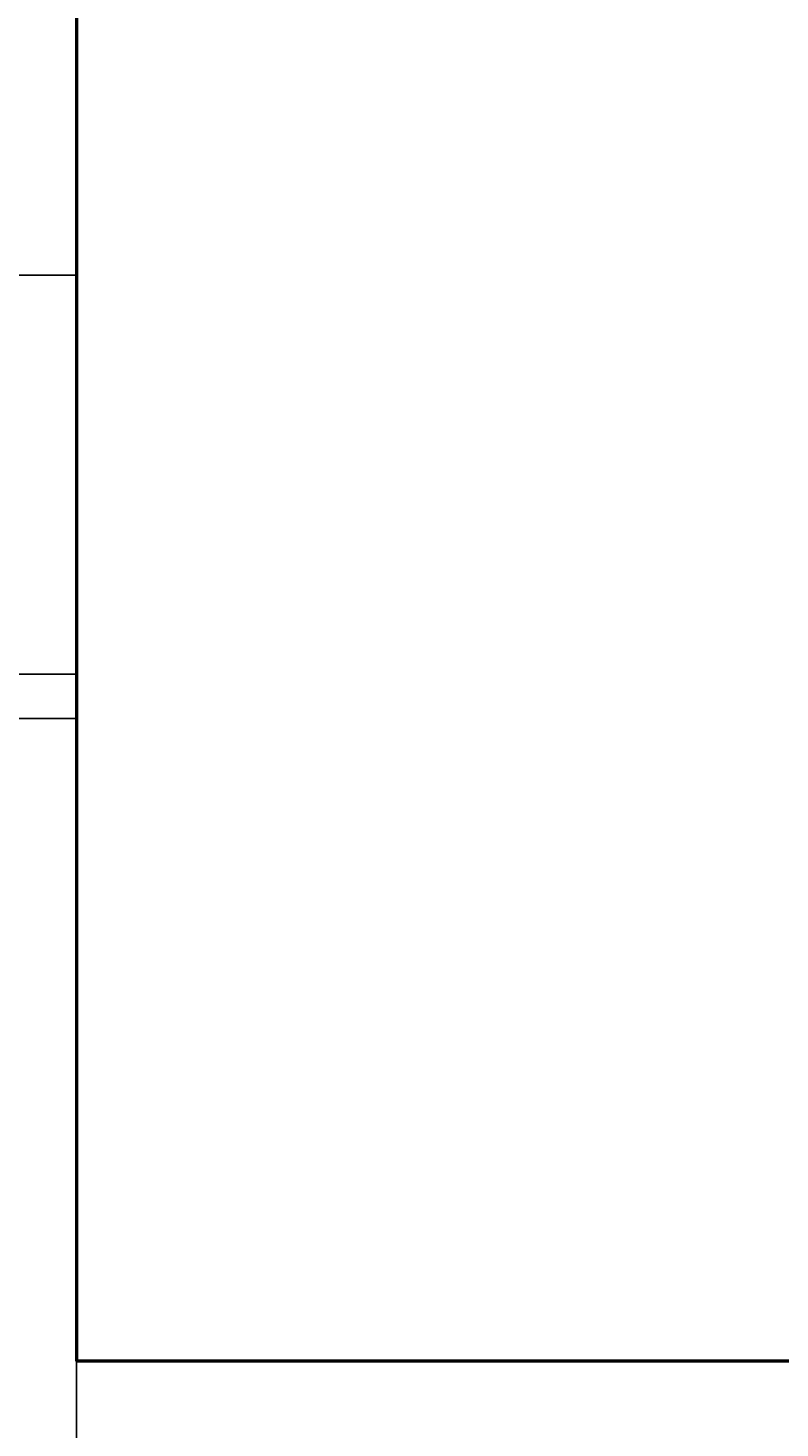
# Model space of a CAD drawing. Units: inches. Extents: x 37 to 824, y -700 to 234.
# Tile 28 of 77: x 168 to 202, y -269 to -206. Entities that reach past the tile are written whole.
import ezdxf

# ---------------------------------------------------------------- set-up
doc = ezdxf.new("R2010")
doc.units = ezdxf.units.IN
doc.header["$MEASUREMENT"] = 0
for name, color, linetype, lineweight in [('A-ANNO-DIMS', 2, 'Continuous', 18), ('A-GLAZ', 4, 'Continuous', 25), ('A-WALL', 2, 'Continuous', 50)]:
    doc.layers.add(name, color=color, linetype=linetype, lineweight=lineweight)
doc.styles.get("Standard").update_dxf_attribs({"font": 'arial.ttf'})
doc.dimstyles.get("Standard").update_dxf_attribs({"dimtxt": 0.18, "dimasz": 0.18, "dimexe": 0.18, "dimexo": 0.0625, "dimgap": 0.09, "dimtad": 0, "dimtih": 1, "dimtoh": 1, "dimdec": 1, "dimzin": 0, "dimdsep": 46, "dimlunit": 4, "dimtxsty": 'Standard', "dimcen": 0.09, "dimadec": 0, "dimazin": 0, "dimtfac": 1, "dimtdec": 1, "dimtofl": 0, "dimtmove": 0, "dimatfit": 3, "dimfxl": 1, "dimtolj": 1, "dimtzin": 0, "dimarcsym": 0})

# ---------------------------------------------------------------- blocks, each defined once
blk = doc.blocks.new('WIN-900')
for p, q in [((0, 9), (0, 0)), ((2, 9), (2, 0)), ((20, 9), (20, 0)), ((38, 9), (38, 0)), ((40, 9), (40, 0)), ((38, 5.5), (2, 5.5)), ((38, 3.5), (2, 3.5))]:
    blk.add_line(p, q)
blk = doc.blocks.new('*D80')
at = {"layer": 'A-ANNO-DIMS', "color": 0, "lineweight": -2, "ltscale": 0.5, "transparency": 16777216}
for p, q in [((170.077, -167.972), (170.077, -400.406)), ((250.19, -167.972), (250.19, -400.406)), ((170.257, -400.226), (209.804, -400.226)), ((250.01, -400.226), (210.463, -400.226))]:
    blk.add_line(p, q, dxfattribs=at)
at = {"layer": 'A-ANNO-DIMS', "color": 0, "ltscale": 0.5, "transparency": 16777216}
for points in [[(170.257, -400.196), (170.257, -400.256), (170.077, -400.226)], [(250.01, -400.196), (250.01, -400.256), (250.19, -400.226)]]:
    blk.add_solid(points, dxfattribs=at)
at = {"layer": 'Defpoints', "color": 0, "ltscale": 0.5, "transparency": 16777216}
for p in [(170.077, -167.91), (250.19, -167.91), (250.19, -400.226)]:
    blk.add_point(p, dxfattribs=at)
at = {"layer": 'A-ANNO-DIMS', "color": 0, "ltscale": 0.5, "transparency": 16777216, "insert": (210.133, -400.226), "char_height": 0.18, "attachment_point": 5}
blk.add_mtext('\\A1;6\'-8"', dxfattribs=at)
blk = doc.blocks.new('*D84')
at = {"layer": 'A-ANNO-DIMS', "color": 0, "lineweight": -2, "ltscale": 0.5, "transparency": 16777216}
for p, q in [((170.077, -265.847), (170.077, 234.17)), ((170.257, 233.99), (189.748, 233.99)), ((209.897, 233.99), (190.406, 233.99)), ((210.077, -265.847), (210.077, 234.17))]:
    blk.add_line(p, q, dxfattribs=at)
at = {"layer": 'A-ANNO-DIMS', "color": 0, "ltscale": 0.5, "transparency": 16777216}
for points in [[(170.257, 234.02), (170.257, 233.96), (170.077, 233.99)], [(209.897, 234.02), (209.897, 233.96), (210.077, 233.99)]]:
    blk.add_solid(points, dxfattribs=at)
at = {"layer": 'Defpoints', "color": 0, "ltscale": 0.5, "transparency": 16777216}
for p in [(210.077, 233.99), (170.077, -265.91), (210.077, -265.91)]:
    blk.add_point(p, dxfattribs=at)
at = {"layer": 'A-ANNO-DIMS', "color": 0, "ltscale": 0.5, "transparency": 16777216, "insert": (190.077, 233.99), "char_height": 0.18, "attachment_point": 5}
blk.add_mtext('\\A1;3\'-4"', dxfattribs=at)
blk = doc.blocks.new('*D85')
at = {"layer": 'A-ANNO-DIMS', "color": 0, "lineweight": -2, "ltscale": 0.5, "transparency": 16777216}
for p, q in [((170.077, -356.847), (170.077, 234.17)), ((170.257, 233.99), (187.748, 233.99)), ((205.897, 233.99), (188.406, 233.99)), ((206.077, -356.847), (206.077, 234.17))]:
    blk.add_line(p, q, dxfattribs=at)
at = {"layer": 'A-ANNO-DIMS', "color": 0, "ltscale": 0.5, "transparency": 16777216}
for points in [[(170.257, 234.02), (170.257, 233.96), (170.077, 233.99)], [(205.897, 234.02), (205.897, 233.96), (206.077, 233.99)]]:
    blk.add_solid(points, dxfattribs=at)
at = {"layer": 'Defpoints', "color": 0, "ltscale": 0.5, "transparency": 16777216}
for p in [(206.077, 233.99), (170.077, -356.91), (206.077, -356.91)]:
    blk.add_point(p, dxfattribs=at)
at = {"layer": 'A-ANNO-DIMS', "color": 0, "ltscale": 0.5, "transparency": 16777216, "insert": (188.077, 233.99), "char_height": 0.18, "attachment_point": 5}
blk.add_mtext('\\A1;3\'-0"', dxfattribs=at)

msp = doc.modelspace()

# ---------------------------------------------------------------- linework, layer by layer
at = {"layer": 'A-WALL'}
for p in [(170.077, -167.91), (290.077, -265.91)]:
    msp.add_line(p, (170.077, -265.91), dxfattribs=at)

# ---------------------------------------------------------------- block references
at = {"layer": 'A-GLAZ', "rotation": 269.9999999999999}
msp.add_blockref('WIN-900', (161.077, -196.909), dxfattribs=at)

# ---------------------------------------------------------------- dimensions: what is measured, and where the dimension line sits
at = {"layer": 'A-ANNO-DIMS', "ltscale": 0.5}
for base, p1, p2, picture, middle in [((210.077, 233.99), (170.077, -265.91), (210.077, -265.91), '*D84', (190.077, 233.99)), ((206.077, 233.99), (170.077, -356.91), (206.077, -356.91), '*D85', (188.077, 233.99)), ((250.19, -400.226), (170.077, -167.91), (250.19, -167.91), '*D80', (210.133, -400.226))]:
    dim = msp.add_linear_dim(base=base, p1=p1, p2=p2, dimstyle='Standard', override={"dimdec": 1, "dimlfac": 1, "dimrnd": 0, "dimzin": 1, "dimdsep": 46, "dimlunit": 4, "dimfrac": 2}, dxfattribs=at)
    dim.commit()
    dim.dimension.update_dxf_attribs({"geometry": picture, "text_midpoint": middle})

doc.saveas('drawing.dxf')
